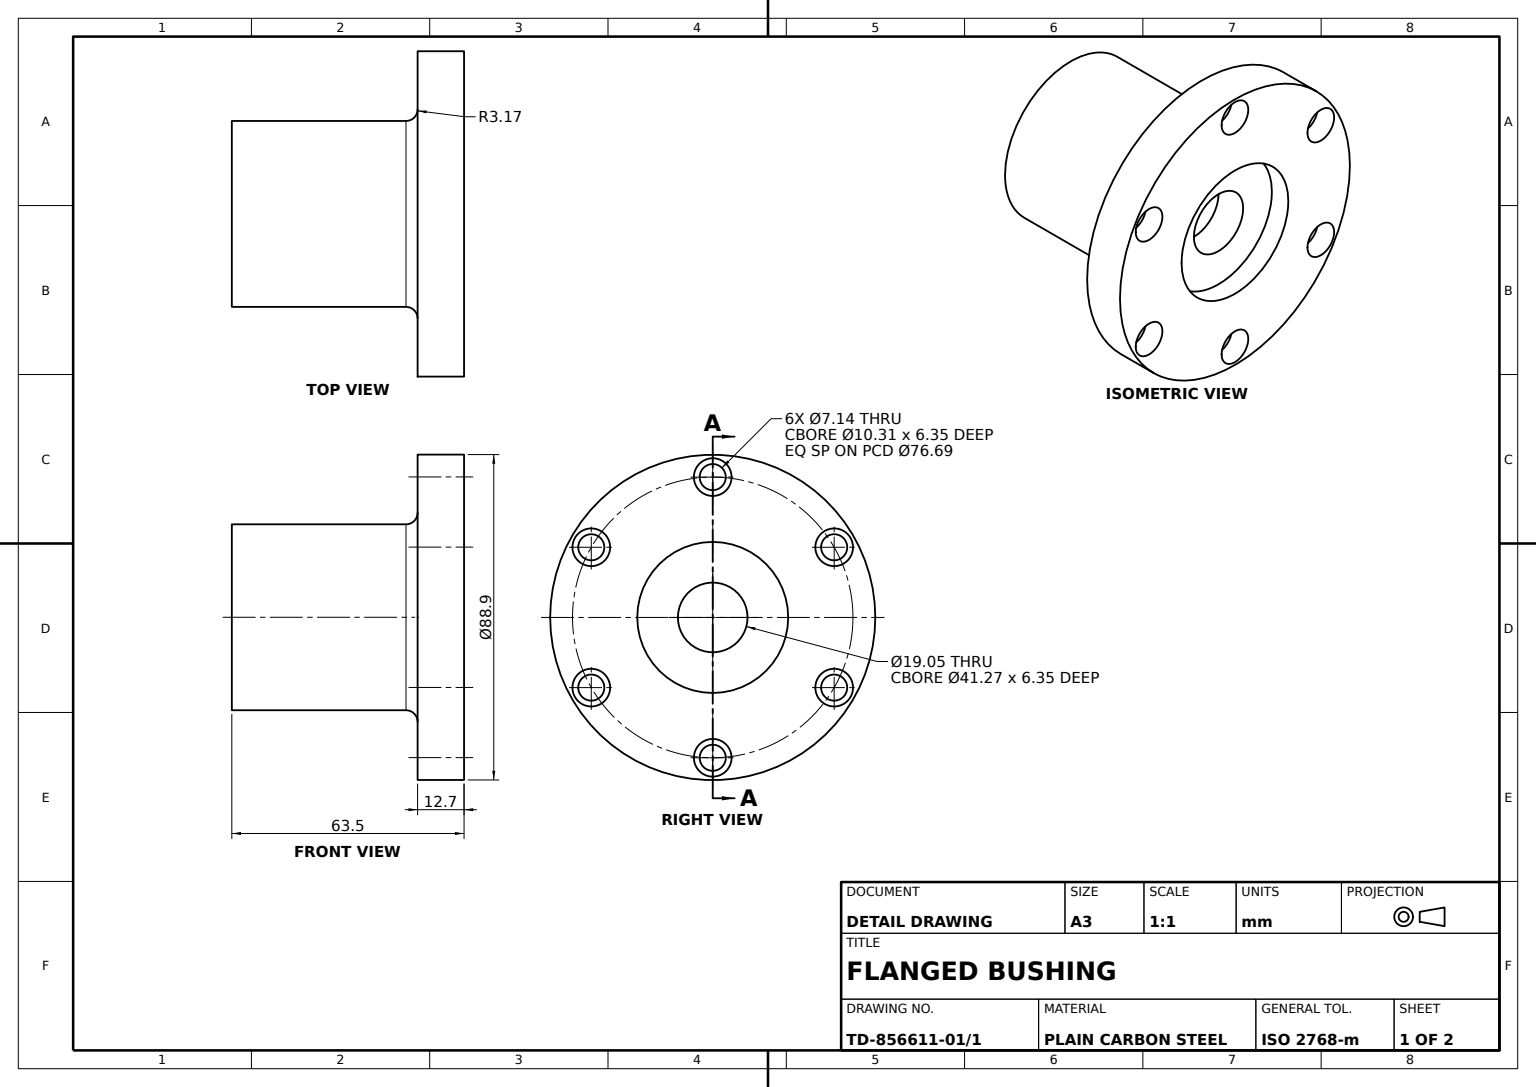
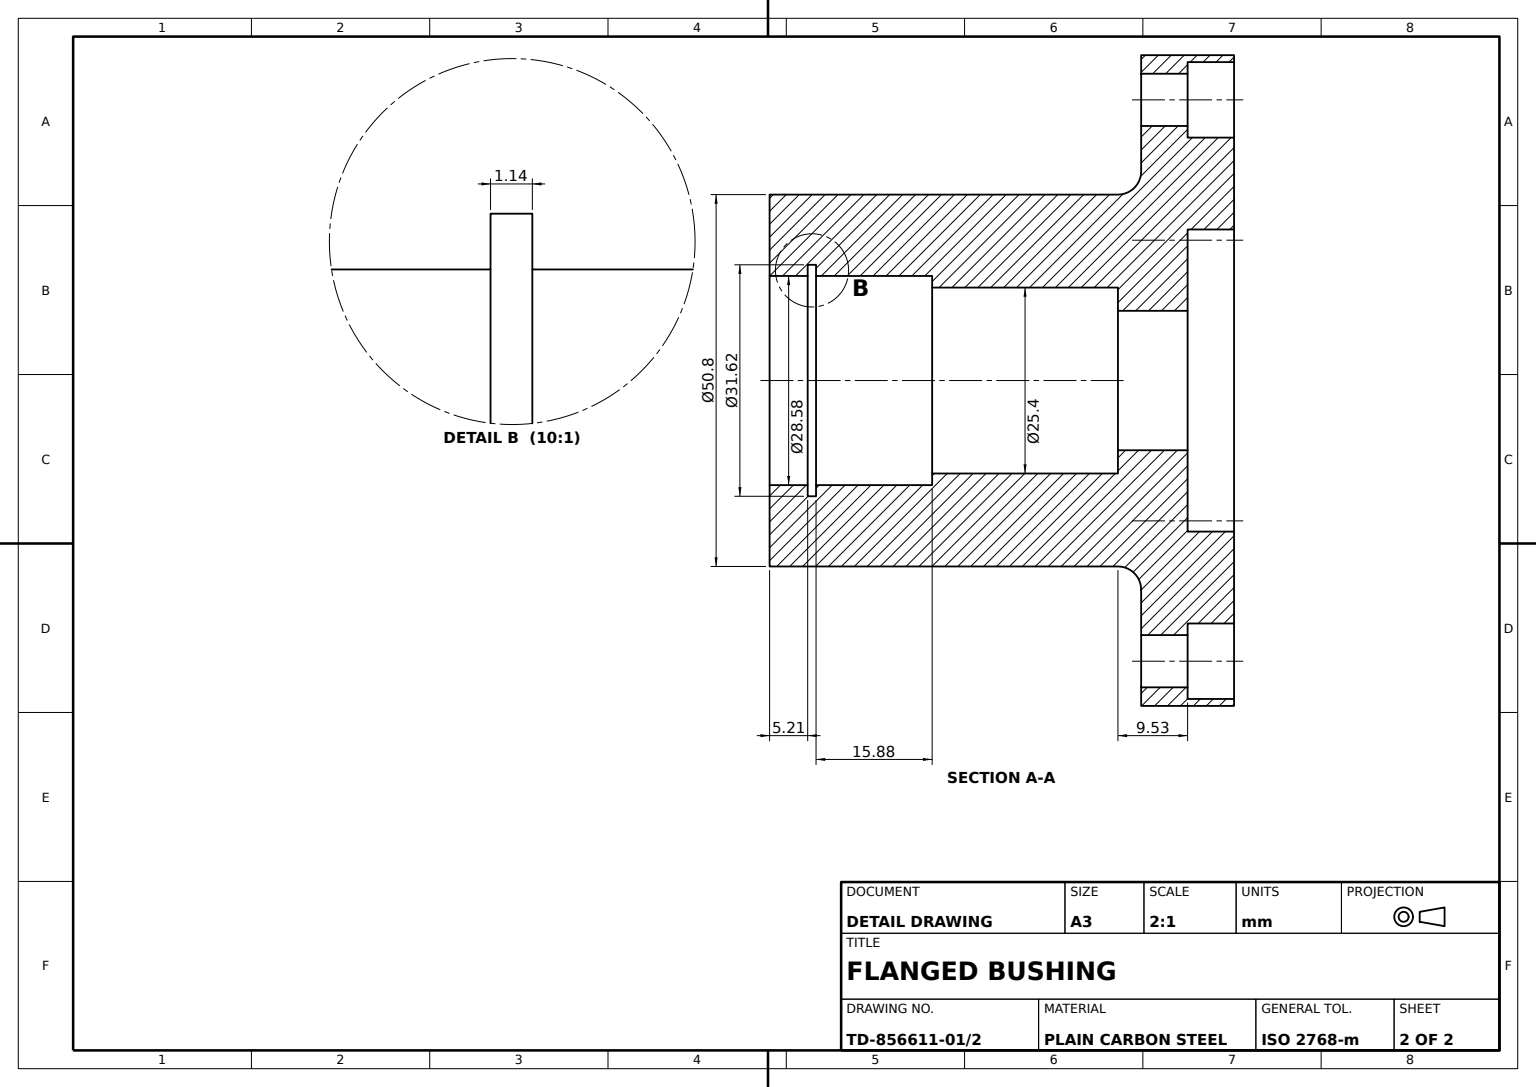
from build123d import *

# Parameters (mm, degrees)
FLANGE_SKETCH_R                   = 44.45
FLANGE_3_5_DEPTH                  = 12.7
HUB_BOSS_SKETCH_R                 = 25.4
HUB_BOSS_2_DEPTH                  = 50.8
REAR_RECESS_SKETCH_R              = 20.6375
REAR_RECESS_1_625_DEPTH           = 6.35
PILOT_BORE_SKETCH_R               = 9.525
PILOT_BORE_0_75_DEPTH             = 9.525
INNER_BORE_SKETCH_R               = 12.7
INNER_BORE_1_0_DEPTH              = 25.4
BEARING_BORE_SKETCH_R             = 14.2875
BEARING_BORE_1_125_DEPTH          = 15.875
RETAINING_GROOVE_SKETCH_R         = 15.8115
RETAINING_RING_GROOVE_1_245_DEPTH = 1.143
THROUGH_BORE_SKETCH_R             = 14.2875
THROUGH_BORE_1_125_DEPTH          = 86.730267986
BOLT_COUNTERBORE_SKETCH_R         = 5.1562
BOLT_COUNTERBORES_6X_0_406_DEPTH  = 6.35
BOLT_HOLE_SKETCH_R                = 3.5687
BOLT_HOLES_6X_0_281_DEPTH         = 85.957209818
HUB_ROOT_FILLET_R0_125_R          = 3.175


with BuildPart() as part:
    # Flange Sketch → Flange Ø3.5 (new body)
    with BuildSketch(Plane.XY):
        Circle(FLANGE_SKETCH_R)
    extrude(amount=FLANGE_3_5_DEPTH)

    # Hub Boss Sketch → Hub Boss Ø2 (add)
    with BuildSketch(Plane.XY.offset(12.7)):
        Circle(HUB_BOSS_SKETCH_R)
    extrude(amount=HUB_BOSS_2_DEPTH)

    # Rear Recess Sketch → Rear Recess Ø1.625 (cut)
    with BuildSketch(Plane(origin=(0, 0, 0), x_dir=(-1, 0, 0), z_dir=(0, 0, -1))):
        Circle(REAR_RECESS_SKETCH_R)
    extrude(amount=-REAR_RECESS_1_625_DEPTH, mode=Mode.SUBTRACT)

    # Pilot Bore Sketch → Pilot Bore Ø0.75 (cut)
    with BuildSketch(Plane(origin=(0, 0, 6.35), x_dir=(-1, 0, 0), z_dir=(0, 0, -1))):
        Circle(PILOT_BORE_SKETCH_R)
    extrude(amount=-PILOT_BORE_0_75_DEPTH, mode=Mode.SUBTRACT)

    # Inner Bore Sketch → Inner Bore Ø1.0 (cut)
    with BuildSketch(Plane(origin=(0, 0, 15.875), x_dir=(-1, 0, 0), z_dir=(0, 0, -1))):
        Circle(INNER_BORE_SKETCH_R)
    extrude(amount=-INNER_BORE_1_0_DEPTH, mode=Mode.SUBTRACT)

    # Bearing Bore Sketch → Bearing Bore Ø1.125 (cut)
    with BuildSketch(Plane(origin=(0, 0, 41.275), x_dir=(-1, 0, 0), z_dir=(0, 0, -1))):
        Circle(BEARING_BORE_SKETCH_R)
    extrude(amount=-BEARING_BORE_1_125_DEPTH, mode=Mode.SUBTRACT)

    # Retaining Groove Sketch → Retaining Ring Groove Ø1.245 (cut)
    with BuildSketch(Plane(origin=(0, 0, 57.15), x_dir=(-1, 0, 0), z_dir=(0, 0, -1))):
        Circle(RETAINING_GROOVE_SKETCH_R)
    extrude(amount=-RETAINING_RING_GROOVE_1_245_DEPTH, mode=Mode.SUBTRACT)

    # Through Bore Sketch → Through Bore Ø1.125 (cut, through all)
    with BuildSketch(Plane(origin=(0, 0, 58.293), x_dir=(-1, 0, 0), z_dir=(0, 0, -1))):
        Circle(THROUGH_BORE_SKETCH_R)
    extrude(amount=-THROUGH_BORE_1_125_DEPTH, mode=Mode.SUBTRACT)

    # Bolt Counterbore Sketch → Bolt Counterbores 6xØ0.406 (cut)
    with BuildSketch(Plane(origin=(0, 0, 0), x_dir=(-1, 0, 0), z_dir=(0, 0, -1))):
        with Locations((0, 38.345083234)):
            Circle(BOLT_COUNTERBORE_SKETCH_R)
        with Locations((33.207816191, 19.172541617)):
            Circle(BOLT_COUNTERBORE_SKETCH_R)
        with Locations((33.207816191, -19.172541617)):
            Circle(BOLT_COUNTERBORE_SKETCH_R)
        with Locations((0, -38.345083234)):
            Circle(BOLT_COUNTERBORE_SKETCH_R)
        with Locations((-33.207816191, -19.172541617)):
            Circle(BOLT_COUNTERBORE_SKETCH_R)
        with Locations((-33.207816191, 19.172541617)):
            Circle(BOLT_COUNTERBORE_SKETCH_R)
    extrude(amount=-BOLT_COUNTERBORES_6X_0_406_DEPTH, mode=Mode.SUBTRACT)

    # Bolt Hole Sketch → Bolt Holes 6xØ0.281 (cut, through all)
    with BuildSketch(Plane(origin=(0, 0, 6.35), x_dir=(-1, 0, 0), z_dir=(0, 0, -1))):
        with Locations((0, 38.345083234)):
            Circle(BOLT_HOLE_SKETCH_R)
        with Locations((33.207816191, 19.172541617)):
            Circle(BOLT_HOLE_SKETCH_R)
        with Locations((33.207816191, -19.172541617)):
            Circle(BOLT_HOLE_SKETCH_R)
        with Locations((0, -38.345083234)):
            Circle(BOLT_HOLE_SKETCH_R)
        with Locations((-33.207816191, -19.172541617)):
            Circle(BOLT_HOLE_SKETCH_R)
        with Locations((-33.207816191, 19.172541617)):
            Circle(BOLT_HOLE_SKETCH_R)
    extrude(amount=-BOLT_HOLES_6X_0_281_DEPTH, mode=Mode.SUBTRACT)

    # Hub Root Fillet R0.125
    hub_root_fillet_r0_125_edges = [part.edges().sort_by_distance(p)[0] for p in [
        (-25.4, 0, 12.7),
    ]]
    fillet(hub_root_fillet_r0_125_edges, radius=HUB_ROOT_FILLET_R0_125_R)


solid = part.part
